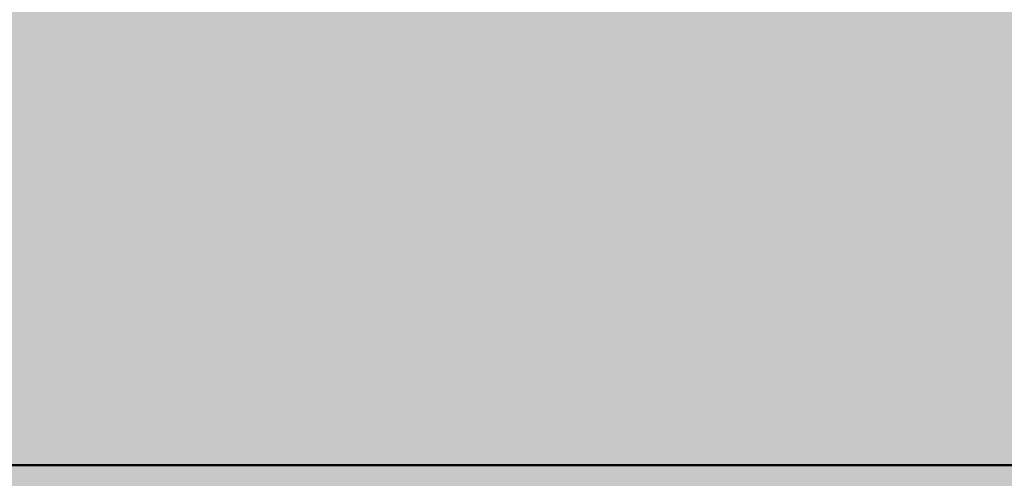
# Model space of a CAD drawing. Units: millimetres. Extents: x 0 to 2267, y 0 to 1823.
# Tile 147 of 256: x 1823.16 to 1833.61, y 1127.28 to 1132.15. Entities that reach past the tile are written whole.
import ezdxf

# ---------------------------------------------------------------- set-up
doc = ezdxf.new("R2010")
doc.units = ezdxf.units.MM
doc.header["$MEASUREMENT"] = 0
for name, color, linetype, lineweight in [('M-DIMS', 2, 'Continuous', 25), ('M-HATC', 252, 'Continuous', 18), ('M-OUTL', 7, 'Continuous', 50)]:
    doc.layers.add(name, color=color, linetype=linetype, lineweight=lineweight)
doc.styles.get("Standard").update_dxf_attribs({"font": 'arial.ttf'})
doc.dimstyles.get("Standard").update_dxf_attribs({"dimtxt": 7, "dimasz": 4, "dimexe": 0.18, "dimexo": 0.0625, "dimgap": 0.09, "dimtad": 0, "dimdec": 0, "dimzin": 0, "dimdsep": 46, "dimtxsty": 'Standard', "dimcen": 0.09, "dimadec": 0, "dimazin": 0, "dimtfac": 1, "dimtdec": 0, "dimtofl": 0, "dimtmove": 0, "dimatfit": 3, "dimfxl": 1, "dimtolj": 1, "dimtzin": 0, "dimarcsym": 0})

# ---------------------------------------------------------------- blocks, each defined once
blk = doc.blocks.new('*D1')
at = {"layer": 'Defpoints', "color": 0, "transparency": 16777216}
for p in [(1593.429, 1127.417), (1843.429, 1127.417), (1843.429, 955.628)]:
    blk.add_point(p, dxfattribs=at)
at = {"layer": 'M-DIMS', "color": 0, "lineweight": -2, "transparency": 16777216}
for p, q in [((1593.429, 1127.355), (1593.429, 955.448)), ((1843.429, 1127.355), (1843.429, 955.448)), ((1597.429, 955.628), (1710.558, 955.628)), ((1839.429, 955.628), (1726.3, 955.628))]:
    blk.add_line(p, q, dxfattribs=at)
at = {"layer": 'M-DIMS', "color": 0, "transparency": 16777216}
for points in [[(1597.429, 956.294), (1597.429, 954.961), (1593.429, 955.628)], [(1839.429, 956.294), (1839.429, 954.961), (1843.429, 955.628)]]:
    blk.add_solid(points, dxfattribs=at)
at = {"layer": 'M-DIMS', "color": 0, "transparency": 16777216, "insert": (1718.429, 955.628), "char_height": 7, "attachment_point": 5}
blk.add_mtext('\\A1;250', dxfattribs=at)

msp = doc.modelspace()

# ---------------------------------------------------------------- hatches: boundary and pattern name
at = {"layer": 'M-HATC'}
h = msp.add_hatch(color=256, dxfattribs=at)
h.dxf.hatch_style = 1
h.paths.add_polyline_path([(2055.771, 1603.062), (1381.087, 1603.062), (1381.087, 1598.062), (2055.771, 1598.062)])
h.paths.add_polyline_path([(2055.771, 1598.062), (1381.087, 1598.062), (1381.087, 1593.062), (2055.771, 1593.062)])
h.paths.add_polyline_path([(2051.307, 1536.761), (1385.55, 1536.761), (1385.55, 1526.761), (1387.55, 1526.761), (1388.537, 1525.053), (1385.332, 1521.233), (1385.332, 1521.223), (2050.254, 1522.749), (2048.321, 1525.053), (2049.307, 1526.761), (2051.307, 1526.761)])
edge = h.paths.add_edge_path()
edge.add_arc((1847.535, 1379.149), 135, 222.60306, 222.89085, ccw=False)
edge.add_line((1748.166, 1287.766), (1683.092, 1287.766))
edge.add_arc((1583.724, 1379.149), 135, 317.10915, 317.39694, ccw=False)
edge.add_arc((1678.969, 1290.671), 5, 222.8909, 317.1091, ccw=False)
edge.add_arc((1774.213, 1379.149), 135, 222.60306, 222.89085, ccw=False)
edge.add_line((1674.845, 1287.766), (1609.771, 1287.766))
edge.add_arc((1510.403, 1379.149), 135, 317.10915, 317.39694, ccw=False)
edge.add_arc((1605.647, 1290.671), 5, 222.8909, 317.1091, ccw=False)
edge.add_arc((1700.892, 1379.149), 135, 222.60306, 222.89085, ccw=False)
edge.add_line((1601.524, 1287.766), (1536.45, 1287.766))
edge.add_arc((1437.081, 1379.149), 135, 317.10915, 317.39694, ccw=False)
edge.add_arc((1532.326, 1290.671), 5, 222.8909, 317.1091, ccw=False)
edge.add_arc((1627.571, 1379.149), 135, 222.60306, 222.89085, ccw=False)
edge.add_line((1528.203, 1287.766), (1505.929, 1287.766))
edge.add_spline(control_points=[(1505.929, 1287.766), (1504.262, 1287.766), (1504.262, 1282.766), (1505.929, 1282.766)], knot_values=[0, 0, 0, 0, 5, 5, 5, 5], degree=3, periodic=0)
edge.add_line((1505.929, 1282.766), (1930.929, 1282.766))
edge.add_spline(control_points=[(1930.929, 1282.766), (1932.596, 1282.766), (1932.596, 1287.766), (1930.929, 1287.766)], knot_values=[0, 0, 0, 0, 5, 5, 5, 5], degree=3, periodic=0)
edge.add_line((1930.929, 1287.766), (1903.056, 1287.766))
edge.add_arc((1803.688, 1379.149), 135, 317.10915, 317.39694, ccw=False)
edge.add_arc((1898.932, 1290.671), 5, 222.8909, 317.1091, ccw=False)
edge.add_arc((1994.177, 1379.149), 135, 222.60306, 222.89085, ccw=False)
edge.add_line((1894.809, 1287.766), (1829.735, 1287.766))
edge.add_arc((1730.366, 1379.149), 135, 317.10915, 317.39694, ccw=False)
edge.add_arc((1825.611, 1290.671), 5, 222.8909, 317.1091, ccw=False)
edge.add_arc((1920.856, 1379.149), 135, 222.60306, 222.89085, ccw=False)
edge.add_line((1821.487, 1287.766), (1756.413, 1287.766))
edge.add_arc((1657.045, 1379.149), 135, 317.10915, 317.39694, ccw=False)
edge.add_arc((1752.29, 1290.671), 5, 222.8909, 317.1091, ccw=False)
edge = h.paths.add_edge_path()
edge.add_spline(control_points=[(1843.429, 1227.247), (1845.096, 1227.247), (1845.096, 1232.247), (1843.429, 1232.247)], knot_values=[0, 0, 0, 0, 5, 5, 5, 5], degree=3, periodic=0)
edge.add_line((1843.429, 1232.247), (1593.429, 1232.247))
edge.add_spline(control_points=[(1593.429, 1232.247), (1591.762, 1232.247), (1591.762, 1227.247), (1593.429, 1227.247)], knot_values=[0, 0, 0, 0, 5, 5, 5, 5], degree=3, periodic=0)
edge.add_line((1593.429, 1227.247), (1843.429, 1227.247))
h.paths.add_polyline_path([(1905.929, 1127.417), (1530.929, 1127.417, 0.414214), (1520.929, 1117.417), (1530.929, 1117.417), (1915.929, 1117.417, 0.414214)])
edge = h.paths.add_edge_path()
edge.add_arc((1397.086, 1498.408), 12.73, 90.7821, 190.8787, ccw=False)
edge.add_line((1396.912, 1511.136), (1428.01, 1511.349))
edge.add_line((1428.01, 1511.349), (1433.01, 1511.349))
edge.add_line((1433.01, 1511.349), (1434.439, 1511.349))
edge.add_arc((1419.474, 1498.08), 20, 41.561, 74.0821)
edge.add_line((1424.959, 1517.314), (1399.935, 1517.256))
edge.add_spline(control_points=[(1399.931, 1517.256), (1399.884, 1517.213), (1399.833, 1517.169), (1399.777, 1517.124)], knot_values=[11.567499, 11.567499, 11.567499, 11.567499, 11.814249, 11.814249, 11.814249, 11.814249], degree=3, periodic=0)
edge.add_spline(control_points=[(1399.633, 1517.01), (1399.583, 1516.972), (1399.531, 1516.934), (1399.476, 1516.895)], knot_values=[11.167718, 11.167718, 11.167718, 11.167718, 11.365188, 11.365188, 11.365188, 11.365188], degree=3, periodic=0)
edge.add_spline(control_points=[(1399.34, 1516.8), (1399.151, 1516.672), (1398.938, 1516.538), (1398.704, 1516.399)], knot_values=[10.376405, 10.376405, 10.376405, 10.376405, 11.00994, 11.00994, 11.00994, 11.00994], degree=3, periodic=0)
edge.add_spline(control_points=[(1398.657, 1516.372), (1398.579, 1516.326), (1398.498, 1516.28), (1398.415, 1516.233)], knot_values=[10.125175, 10.125175, 10.125175, 10.125175, 10.334406, 10.334406, 10.334406, 10.334406], degree=3, periodic=0)
edge.add_spline(control_points=[(1398.264, 1516.149), (1398.196, 1516.111), (1398.126, 1516.073), (1398.055, 1516.035)], knot_values=[9.832246, 9.832246, 9.832246, 9.832246, 9.999658, 9.999658, 9.999658, 9.999658], degree=3, periodic=0)
edge.add_spline(control_points=[(1397.999, 1516.005), (1397.731, 1515.862), (1397.446, 1515.717), (1397.147, 1515.571)], knot_values=[9.161808, 9.161808, 9.161808, 9.161808, 9.787769, 9.787769, 9.787769, 9.787769], degree=3, periodic=0)
edge.add_spline(control_points=[(1397.147, 1515.571), (1396.842, 1515.423), (1396.522, 1515.274), (1396.191, 1515.126)], knot_values=[8.524455, 8.524455, 8.524455, 8.524455, 9.161808, 9.161808, 9.161808, 9.161808], degree=3, periodic=0)
edge.add_spline(control_points=[(1396.078, 1515.076), (1395.985, 1515.035), (1395.892, 1514.994), (1395.798, 1514.953)], knot_values=[8.275193, 8.275193, 8.275193, 8.275193, 8.451726, 8.451726, 8.451726, 8.451726], degree=3, periodic=0)
edge.add_spline(control_points=[(1395.602, 1514.869), (1395.5, 1514.826), (1395.397, 1514.782), (1395.293, 1514.739)], knot_values=[7.962917, 7.962917, 7.962917, 7.962917, 8.152764, 8.152764, 8.152764, 8.152764], degree=3, periodic=0)
edge.add_spline(control_points=[(1395.212, 1514.706), (1394.828, 1514.547), (1394.435, 1514.393), (1394.036, 1514.244)], knot_values=[7.21254, 7.21254, 7.21254, 7.21254, 7.913148, 7.913148, 7.913148, 7.913148], degree=3, periodic=0)
edge.add_spline(control_points=[(1394.036, 1514.244), (1393.708, 1514.121), (1393.375, 1514.003), (1393.043, 1513.889)], knot_values=[6.633733, 6.633733, 6.633733, 6.633733, 7.21254, 7.21254, 7.21254, 7.21254], degree=3, periodic=0)
edge.add_spline(control_points=[(1392.821, 1513.815), (1392.72, 1513.781), (1392.618, 1513.748), (1392.517, 1513.715)], knot_values=[6.328796, 6.328796, 6.328796, 6.328796, 6.505493, 6.505493, 6.505493, 6.505493], degree=3, periodic=0)
edge.add_spline(control_points=[(1392.517, 1513.715), (1392.319, 1513.652), (1392.121, 1513.59), (1391.924, 1513.531)], knot_values=[5.984605, 5.984605, 5.984605, 5.984605, 6.328796, 6.328796, 6.328796, 6.328796], degree=3, periodic=0)
edge.add_spline(control_points=[(1391.792, 1513.491), (1391.312, 1513.35), (1390.838, 1513.224), (1390.378, 1513.117)], knot_values=[5.066697, 5.066697, 5.066697, 5.066697, 5.907055, 5.907055, 5.907055, 5.907055], degree=3, periodic=0)
edge.add_spline(control_points=[(1390.378, 1513.117), (1390.18, 1513.071), (1389.984, 1513.028), (1389.791, 1512.99)], knot_values=[4.70367, 4.70367, 4.70367, 4.70367, 5.066695, 5.066695, 5.066695, 5.066695], degree=3, periodic=0)
edge.add_spline(control_points=[(1389.422, 1512.92), (1389.246, 1512.889), (1389.073, 1512.862), (1388.904, 1512.838)], knot_values=[4.130571, 4.130571, 4.130571, 4.130571, 4.469816, 4.469816, 4.469816, 4.469816], degree=3, periodic=0)
edge.add_spline(control_points=[(1388.904, 1512.838), (1388.591, 1512.795), (1388.291, 1512.764), (1388.007, 1512.749)], knot_values=[3.504031, 3.504031, 3.504031, 3.504031, 4.130571, 4.130571, 4.130571, 4.130571], degree=3, periodic=0)
edge.add_spline(control_points=[(1387.936, 1512.746), (1387.854, 1512.742), (1387.773, 1512.74), (1387.694, 1512.739)], knot_values=[3.268866, 3.268866, 3.268866, 3.268866, 3.451164, 3.451164, 3.451164, 3.451164], degree=3, periodic=0)
edge.add_spline(control_points=[(1387.335, 1512.744), (1387.208, 1512.75), (1387.085, 1512.76), (1386.967, 1512.774)], knot_values=[2.670686, 2.670686, 2.670686, 2.670686, 2.984, 2.984, 2.984, 2.984], degree=3, periodic=0)
edge.add_spline(control_points=[(1386.833, 1512.792), (1386.821, 1512.794), (1386.809, 1512.796), (1386.797, 1512.798)], knot_values=[2.516981, 2.516981, 2.516981, 2.516981, 2.549528, 2.549528, 2.549528, 2.549528], degree=3, periodic=0)
edge.add_spline(control_points=[(1386.453, 1512.873), (1386.426, 1512.881), (1386.399, 1512.889), (1386.373, 1512.897)], knot_values=[2.095869, 2.095869, 2.095869, 2.095869, 2.17941, 2.17941, 2.17941, 2.17941], degree=3, periodic=0)
edge.add_spline(control_points=[(1386.069, 1513.019), (1386.063, 1513.022), (1386.058, 1513.025), (1386.052, 1513.028)], knot_values=[1.72453, 1.72453, 1.72453, 1.72453, 1.745933, 1.745933, 1.745933, 1.745933], degree=3, periodic=0)
edge.add_arc((1399.474, 1498.08), 20, 131.8243, 180)
edge.add_arc((1630.334, 1505.548), 250.971, 181.70518, 236.42798)
edge.add_arc((1605.34, 1483.304), 218.782, 238.66083, 243.34961)
edge.add_arc((1647.091, 1510.359), 262.899, 183.12984, 237.85344, ccw=False)
h.paths.add_polyline_path([(1406.537, 1391.964, 0.149382), (1491.551, 1296.442, -0.129517)], flags=17)
edge = h.paths.add_edge_path()
edge.add_arc((2037.384, 1498.08), 20, 0, 48.2659)
edge.add_spline(control_points=[(2050.697, 1513.005), (2050.651, 1512.985), (2050.603, 1512.966), (2050.554, 1512.948)], knot_values=[1.835652, 1.835652, 1.835652, 1.835652, 2.000781, 2.000781, 2.000781, 2.000781], degree=3, periodic=0)
edge.add_spline(control_points=[(2050.462, 1512.917), (2050.479, 1512.922), (2050.496, 1512.928), (2050.513, 1512.934)], knot_values=[2.045477, 2.045477, 2.045477, 2.045477, 2.101389, 2.101389, 2.101389, 2.101389], degree=3, periodic=0)
edge.add_spline(control_points=[(2050.129, 1512.834), (2050.198, 1512.847), (2050.266, 1512.862), (2050.331, 1512.879)], knot_values=[2.237629, 2.237629, 2.237629, 2.237629, 2.435841, 2.435841, 2.435841, 2.435841], degree=3, periodic=0)
edge.add_spline(control_points=[(2050.095, 1512.828), (2050.106, 1512.83), (2050.118, 1512.832), (2050.129, 1512.834)], knot_values=[2.435841, 2.435841, 2.435841, 2.435841, 2.468321, 2.468321, 2.468321, 2.468321], degree=3, periodic=0)
edge.add_spline(control_points=[(2049.784, 1512.785), (2049.855, 1512.792), (2049.924, 1512.801), (2049.992, 1512.811)], knot_values=[2.563852, 2.563852, 2.563852, 2.563852, 2.748541, 2.748541, 2.748541, 2.748541], degree=3, periodic=0)
edge.add_spline(control_points=[(2049.405, 1512.762), (2049.536, 1512.765), (2049.663, 1512.773), (2049.784, 1512.785)], knot_values=[2.748541, 2.748541, 2.748541, 2.748541, 3.064882, 3.064882, 3.064882, 3.064882], degree=3, periodic=0)
edge.add_spline(control_points=[(2049.17, 1512.76), (2049.234, 1512.759), (2049.297, 1512.759), (2049.358, 1512.761)], knot_values=[3.102309, 3.102309, 3.102309, 3.102309, 3.2503, 3.2503, 3.2503, 3.2503], degree=3, periodic=0)
edge.add_spline(control_points=[(2048.857, 1512.769), (2048.964, 1512.764), (2049.068, 1512.761), (2049.17, 1512.76)], knot_values=[3.2503, 3.2503, 3.2503, 3.2503, 3.486069, 3.486069, 3.486069, 3.486069], degree=3, periodic=0)
edge.add_spline(control_points=[(2048.692, 1512.779), (2048.373, 1512.801), (2048.035, 1512.841), (2047.682, 1512.897)], knot_values=[3.606429, 3.606429, 3.606429, 3.606429, 4.2989, 4.2989, 4.2989, 4.2989], degree=3, periodic=0)
edge.add_spline(control_points=[(2047.682, 1512.897), (2047.546, 1512.919), (2047.408, 1512.942), (2047.268, 1512.969)], knot_values=[4.2989, 4.2989, 4.2989, 4.2989, 4.565769, 4.565769, 4.565769, 4.565769], degree=3, periodic=0)
edge.add_spline(control_points=[(2047.268, 1512.969), (2047.145, 1512.991), (2047.021, 1513.016), (2046.895, 1513.042)], knot_values=[4.565769, 4.565769, 4.565769, 4.565769, 4.799971, 4.799971, 4.799971, 4.799971], degree=3, periodic=0)
edge.add_spline(control_points=[(2046.895, 1513.042), (2046.529, 1513.119), (2046.151, 1513.209), (2045.768, 1513.311)], knot_values=[4.799971, 4.799971, 4.799971, 4.799971, 5.483718, 5.483718, 5.483718, 5.483718], degree=3, periodic=0)
edge.add_spline(control_points=[(2045.768, 1513.311), (2045.372, 1513.415), (2044.97, 1513.532), (2044.566, 1513.659)], knot_values=[5.483718, 5.483718, 5.483718, 5.483718, 6.187866, 6.187866, 6.187866, 6.187866], degree=3, periodic=0)
edge.add_spline(control_points=[(2044.566, 1513.659), (2044.415, 1513.706), (2044.263, 1513.755), (2044.112, 1513.805)], knot_values=[6.187866, 6.187866, 6.187866, 6.187866, 6.451551, 6.451551, 6.451551, 6.451551], degree=3, periodic=0)
edge.add_spline(control_points=[(2044.112, 1513.805), (2043.997, 1513.843), (2043.882, 1513.881), (2043.767, 1513.92)], knot_values=[6.451551, 6.451551, 6.451551, 6.451551, 6.651434, 6.651434, 6.651434, 6.651434], degree=3, periodic=0)
edge.add_spline(control_points=[(2043.767, 1513.92), (2043.372, 1514.055), (2042.977, 1514.198), (2042.589, 1514.346)], knot_values=[6.651434, 6.651434, 6.651434, 6.651434, 7.338879, 7.338879, 7.338879, 7.338879], degree=3, periodic=0)
edge.add_spline(control_points=[(2042.589, 1514.346), (2042.164, 1514.507), (2041.746, 1514.675), (2041.341, 1514.846)], knot_values=[7.338879, 7.338879, 7.338879, 7.338879, 8.089209, 8.089209, 8.089209, 8.089209], degree=3, periodic=0)
edge.add_spline(control_points=[(2041.341, 1514.846), (2041.103, 1514.946), (2040.869, 1515.048), (2040.64, 1515.15)], knot_values=[8.089209, 8.089209, 8.089209, 8.089209, 8.529587, 8.529587, 8.529587, 8.529587], degree=3, periodic=0)
edge.add_spline(control_points=[(2040.51, 1515.209), (2040.082, 1515.402), (2039.675, 1515.597), (2039.295, 1515.789)], knot_values=[8.613818, 8.613818, 8.613818, 8.613818, 9.44571, 9.44571, 9.44571, 9.44571], degree=3, periodic=0)
edge.add_spline(control_points=[(2039.295, 1515.789), (2039.062, 1515.907), (2038.839, 1516.025), (2038.629, 1516.14)], knot_values=[9.44571, 9.44571, 9.44571, 9.44571, 9.956404, 9.956404, 9.956404, 9.956404], degree=3, periodic=0)
edge.add_spline(control_points=[(2038.629, 1516.14), (2038.519, 1516.2), (2038.412, 1516.26), (2038.309, 1516.319)], knot_values=[9.956404, 9.956404, 9.956404, 9.956404, 10.223542, 10.223542, 10.223542, 10.223542], degree=3, periodic=0)
edge.add_spline(control_points=[(2038.309, 1516.319), (2038.214, 1516.374), (2038.122, 1516.428), (2038.033, 1516.481)], knot_values=[10.223542, 10.223542, 10.223542, 10.223542, 10.47051, 10.47051, 10.47051, 10.47051], degree=3, periodic=0)
edge.add_spline(control_points=[(2038.033, 1516.481), (2037.786, 1516.63), (2037.564, 1516.773), (2037.372, 1516.909)], knot_values=[10.47051, 10.47051, 10.47051, 10.47051, 11.15767, 11.15767, 11.15767, 11.15767], degree=3, periodic=0)
edge.add_spline(control_points=[(2037.372, 1516.909), (2037.279, 1516.975), (2037.193, 1517.04), (2037.114, 1517.102)], knot_values=[11.15767, 11.15767, 11.15767, 11.15767, 11.49227, 11.49227, 11.49227, 11.49227], degree=3, periodic=0)
edge.add_spline(control_points=[(2036.856, 1517.326), (2036.915, 1517.269), (2036.981, 1517.21), (2037.056, 1517.149)], knot_values=[11.577341, 11.577341, 11.577341, 11.577341, 11.91035, 11.91035, 11.91035, 11.91035], degree=3, periodic=0)
edge.add_spline(control_points=[(2036.807, 1517.375), (2036.823, 1517.359), (2036.839, 1517.342), (2036.856, 1517.326)], knot_values=[11.91035, 11.91035, 11.91035, 11.91035, 12.007402, 12.007402, 12.007402, 12.007402], degree=3, periodic=0)
edge.add_spline(control_points=[(2036.702, 1517.494), (2036.71, 1517.483), (2036.72, 1517.472), (2036.729, 1517.461)], knot_values=[12.184155, 12.184155, 12.184155, 12.184155, 12.255409, 12.255409, 12.255409, 12.255409], degree=3, periodic=0)
edge.add_spline(control_points=[(2036.616, 1517.621), (2036.62, 1517.613), (2036.624, 1517.606), (2036.629, 1517.598)], knot_values=[12.487913, 12.487913, 12.487913, 12.487913, 12.541035, 12.541035, 12.541035, 12.541035], degree=3, periodic=0)
edge.add_spline(control_points=[(2036.563, 1517.786), (2036.564, 1517.779), (2036.564, 1517.773), (2036.565, 1517.766)], knot_values=[12.911761, 12.911761, 12.911761, 12.911761, 12.968286, 12.968286, 12.968286, 12.968286], degree=3, periodic=0)
edge.add_spline(control_points=[(2036.617, 1517.93), (2036.612, 1517.926), (2036.609, 1517.921), (2036.605, 1517.916)], knot_values=[13.382527, 13.382527, 13.382527, 13.382527, 13.433791, 13.433791, 13.433791, 13.433791], degree=3, periodic=0)
edge.add_spline(control_points=[(2036.749, 1518.017), (2036.736, 1518.012), (2036.724, 1518.006), (2036.712, 1518)], knot_values=[13.726299, 13.726299, 13.726299, 13.726299, 13.809928, 13.809928, 13.809928, 13.809928], degree=3, periodic=0)
edge.add_spline(control_points=[(2036.86, 1518.053), (2036.839, 1518.047), (2036.818, 1518.042), (2036.799, 1518.035)], knot_values=[13.910887, 13.910887, 13.910887, 13.910887, 14.02153, 14.02153, 14.02153, 14.02153], degree=3, periodic=0)
edge.add_line((2036.964, 1518.08), (2032.384, 1518.08))
edge.add_line((2032.384, 1518.08), (2027.384, 1518.08))
edge.add_line((2027.384, 1518.08), (2022.384, 1518.08))
edge.add_line((2022.384, 1518.08), (2017.384, 1518.08))
edge.add_arc((2017.384, 1498.08), 20, 90, 138.439)
edge.add_line((2002.419, 1511.349), (2003.848, 1511.349))
edge.add_line((2003.848, 1511.349), (2008.848, 1511.349))
edge.add_line((2008.848, 1511.349), (2039.772, 1511.138))
edge.add_arc((2039.772, 1498.408), 12.73, -10.8787, 90, ccw=False)
edge.add_arc((1789.767, 1510.359), 262.899, 302.14656, 356.87016, ccw=False)
edge.add_arc((1831.518, 1483.304), 218.782, 296.65039, 301.33917)
edge.add_arc((1806.524, 1505.548), 250.971, 303.57202, 358.29482)
h.paths.add_polyline_path([(2030.321, 1391.964, -0.129517), (1945.307, 1296.442, 0.149382)], flags=17)
edge = h.paths.add_edge_path()
edge.add_spline(control_points=[(2037.246, 1518.082), (2037.29, 1518.081), (2037.336, 1518.08), (2037.384, 1518.08)], knot_values=[0.000012, 0.000012, 0.000012, 0.000012, 0.144754, 0.144754, 0.144754, 0.144754], degree=3, periodic=0)
edge.add_line((2037.336, 1518.08), (2037.01, 1518.08))
edge.add_spline(control_points=[(2037.01, 1518.08), (2036.982, 1518.077), (2036.956, 1518.073), (2036.931, 1518.068)], knot_values=[14.13465, 14.13465, 14.13465, 14.13465, 14.247197, 14.247197, 14.247197, 14.247197], degree=3, periodic=0)
edge.add_spline(control_points=[(2036.931, 1518.068), (2036.928, 1518.067), (2036.924, 1518.067), (2036.921, 1518.066)], knot_values=[14.118315, 14.118315, 14.118315, 14.118315, 14.13465, 14.13465, 14.13465, 14.13465], degree=3, periodic=0)
edge.add_spline(control_points=[(2036.921, 1518.066), (2036.912, 1518.064), (2036.903, 1518.063), (2036.895, 1518.061)], knot_values=[14.078086, 14.078086, 14.078086, 14.078086, 14.118315, 14.118315, 14.118315, 14.118315], degree=3, periodic=0)
edge.add_spline(control_points=[(2036.895, 1518.061), (2036.883, 1518.058), (2036.872, 1518.056), (2036.86, 1518.053)], knot_values=[14.02153, 14.02153, 14.02153, 14.02153, 14.078086, 14.078086, 14.078086, 14.078086], degree=3, periodic=0)
edge.add_spline(control_points=[(2036.86, 1518.053), (2036.839, 1518.047), (2036.818, 1518.042), (2036.799, 1518.035)], knot_values=[13.910887, 13.910887, 13.910887, 13.910887, 14.02153, 14.02153, 14.02153, 14.02153], degree=3, periodic=0)
edge.add_spline(control_points=[(2036.799, 1518.035), (2036.798, 1518.035), (2036.797, 1518.035), (2036.797, 1518.035)], knot_values=[13.906906, 13.906906, 13.906906, 13.906906, 13.910887, 13.910887, 13.910887, 13.910887], degree=3, periodic=0)
edge.add_spline(control_points=[(2036.797, 1518.035), (2036.788, 1518.032), (2036.78, 1518.029), (2036.772, 1518.026)], knot_values=[13.857826, 13.857826, 13.857826, 13.857826, 13.906906, 13.906906, 13.906906, 13.906906], degree=3, periodic=0)
edge.add_spline(control_points=[(2036.772, 1518.026), (2036.764, 1518.023), (2036.756, 1518.02), (2036.749, 1518.017)], knot_values=[13.809928, 13.809928, 13.809928, 13.809928, 13.857826, 13.857826, 13.857826, 13.857826], degree=3, periodic=0)
edge.add_spline(control_points=[(2036.749, 1518.017), (2036.736, 1518.012), (2036.724, 1518.006), (2036.712, 1518)], knot_values=[13.726299, 13.726299, 13.726299, 13.726299, 13.809928, 13.809928, 13.809928, 13.809928], degree=3, periodic=0)
edge.add_spline(control_points=[(2036.712, 1518), (2036.712, 1518), (2036.712, 1518), (2036.711, 1518)], knot_values=[13.723993, 13.723993, 13.723993, 13.723993, 13.726299, 13.726299, 13.726299, 13.726299], degree=3, periodic=0)
edge.add_spline(control_points=[(2036.711, 1518), (2036.706, 1517.997), (2036.701, 1517.994), (2036.696, 1517.992)], knot_values=[13.686536, 13.686536, 13.686536, 13.686536, 13.723993, 13.723993, 13.723993, 13.723993], degree=3, periodic=0)
edge.add_spline(control_points=[(2036.696, 1517.992), (2036.692, 1517.989), (2036.687, 1517.987), (2036.683, 1517.984)], knot_values=[13.651251, 13.651251, 13.651251, 13.651251, 13.686536, 13.686536, 13.686536, 13.686536], degree=3, periodic=0)
edge.add_spline(control_points=[(2036.683, 1517.984), (2036.676, 1517.98), (2036.67, 1517.976), (2036.664, 1517.971)], knot_values=[13.596804, 13.596804, 13.596804, 13.596804, 13.651251, 13.651251, 13.651251, 13.651251], degree=3, periodic=0)
edge.add_spline(control_points=[(2036.664, 1517.971), (2036.664, 1517.971), (2036.663, 1517.971), (2036.663, 1517.971)], knot_values=[13.593956, 13.593956, 13.593956, 13.593956, 13.596804, 13.596804, 13.596804, 13.596804], degree=3, periodic=0)
edge.add_spline(control_points=[(2036.663, 1517.971), (2036.66, 1517.969), (2036.658, 1517.967), (2036.655, 1517.965)], knot_values=[13.570322, 13.570322, 13.570322, 13.570322, 13.593956, 13.593956, 13.593956, 13.593956], degree=3, periodic=0)
edge.add_spline(control_points=[(2036.655, 1517.965), (2036.653, 1517.963), (2036.65, 1517.961), (2036.647, 1517.959)], knot_values=[13.545477, 13.545477, 13.545477, 13.545477, 13.570322, 13.570322, 13.570322, 13.570322], degree=3, periodic=0)
edge.add_spline(control_points=[(2036.647, 1517.959), (2036.647, 1517.959), (2036.647, 1517.959), (2036.647, 1517.959)], knot_values=[13.543931, 13.543931, 13.543931, 13.543931, 13.545477, 13.545477, 13.545477, 13.545477], degree=3, periodic=0)
edge.add_spline(control_points=[(2036.647, 1517.959), (2036.641, 1517.954), (2036.636, 1517.949), (2036.631, 1517.945)], knot_values=[13.488237, 13.488237, 13.488237, 13.488237, 13.543931, 13.543931, 13.543931, 13.543931], degree=3, periodic=0)
edge.add_spline(control_points=[(2036.631, 1517.945), (2036.628, 1517.942), (2036.626, 1517.94), (2036.623, 1517.937)], knot_values=[13.460307, 13.460307, 13.460307, 13.460307, 13.488237, 13.488237, 13.488237, 13.488237], degree=3, periodic=0)
edge.add_spline(control_points=[(2036.623, 1517.937), (2036.622, 1517.936), (2036.62, 1517.934), (2036.618, 1517.932)], knot_values=[13.439712, 13.439712, 13.439712, 13.439712, 13.460307, 13.460307, 13.460307, 13.460307], degree=3, periodic=0)
edge.add_spline(control_points=[(2036.618, 1517.932), (2036.618, 1517.931), (2036.617, 1517.931), (2036.617, 1517.93)], knot_values=[13.433791, 13.433791, 13.433791, 13.433791, 13.439712, 13.439712, 13.439712, 13.439712], degree=3, periodic=0)
edge.add_spline(control_points=[(2036.617, 1517.93), (2036.612, 1517.926), (2036.609, 1517.921), (2036.605, 1517.916)], knot_values=[13.382527, 13.382527, 13.382527, 13.382527, 13.433791, 13.433791, 13.433791, 13.433791], degree=3, periodic=0)
edge.add_spline(control_points=[(2036.605, 1517.916), (2036.603, 1517.913), (2036.6, 1517.91), (2036.598, 1517.907)], knot_values=[13.350017, 13.350017, 13.350017, 13.350017, 13.382527, 13.382527, 13.382527, 13.382527], degree=3, periodic=0)
edge.add_spline(control_points=[(2036.598, 1517.907), (2036.597, 1517.906), (2036.596, 1517.904), (2036.595, 1517.903)], knot_values=[13.333922, 13.333922, 13.333922, 13.333922, 13.350017, 13.350017, 13.350017, 13.350017], degree=3, periodic=0)
edge.add_spline(control_points=[(2036.595, 1517.903), (2036.595, 1517.902), (2036.594, 1517.901), (2036.593, 1517.9)], knot_values=[13.323828, 13.323828, 13.323828, 13.323828, 13.333922, 13.333922, 13.333922, 13.333922], degree=3, periodic=0)
edge.add_spline(control_points=[(2036.593, 1517.9), (2036.59, 1517.895), (2036.588, 1517.891), (2036.585, 1517.886)], knot_values=[13.277545, 13.277545, 13.277545, 13.277545, 13.323828, 13.323828, 13.323828, 13.323828], degree=3, periodic=0)
edge.add_spline(control_points=[(2036.585, 1517.886), (2036.584, 1517.883), (2036.582, 1517.879), (2036.58, 1517.875)], knot_values=[13.240119, 13.240119, 13.240119, 13.240119, 13.277545, 13.277545, 13.277545, 13.277545], degree=3, periodic=0)
edge.add_spline(control_points=[(2036.58, 1517.875), (2036.58, 1517.874), (2036.579, 1517.873), (2036.578, 1517.872)], knot_values=[13.228211, 13.228211, 13.228211, 13.228211, 13.240119, 13.240119, 13.240119, 13.240119], degree=3, periodic=0)
edge.add_spline(control_points=[(2036.578, 1517.872), (2036.578, 1517.87), (2036.577, 1517.869), (2036.577, 1517.868)], knot_values=[13.215717, 13.215717, 13.215717, 13.215717, 13.228211, 13.228211, 13.228211, 13.228211], degree=3, periodic=0)
edge.add_spline(control_points=[(2036.577, 1517.868), (2036.575, 1517.864), (2036.574, 1517.86), (2036.573, 1517.857)], knot_values=[13.179847, 13.179847, 13.179847, 13.179847, 13.215717, 13.215717, 13.215717, 13.215717], degree=3, periodic=0)
edge.add_spline(control_points=[(2036.573, 1517.857), (2036.571, 1517.851), (2036.57, 1517.846), (2036.569, 1517.841)], knot_values=[13.132017, 13.132017, 13.132017, 13.132017, 13.179847, 13.179847, 13.179847, 13.179847], degree=3, periodic=0)
edge.add_spline(control_points=[(2036.569, 1517.841), (2036.568, 1517.84), (2036.568, 1517.839), (2036.568, 1517.838)], knot_values=[13.122482, 13.122482, 13.122482, 13.122482, 13.132017, 13.132017, 13.132017, 13.132017], degree=3, periodic=0)
edge.add_spline(control_points=[(2036.568, 1517.838), (2036.568, 1517.836), (2036.567, 1517.835), (2036.567, 1517.833)], knot_values=[13.105592, 13.105592, 13.105592, 13.105592, 13.122482, 13.122482, 13.122482, 13.122482], degree=3, periodic=0)
edge.add_spline(control_points=[(2036.567, 1517.833), (2036.566, 1517.829), (2036.566, 1517.826), (2036.565, 1517.822)], knot_values=[13.074063, 13.074063, 13.074063, 13.074063, 13.105592, 13.105592, 13.105592, 13.105592], degree=3, periodic=0)
edge.add_spline(control_points=[(2036.565, 1517.822), (2036.565, 1517.822), (2036.565, 1517.822), (2036.565, 1517.822)], knot_values=[13.074043, 13.074043, 13.074043, 13.074043, 13.074063, 13.074063, 13.074063, 13.074063], degree=3, periodic=0)
edge.add_spline(control_points=[(2036.565, 1517.822), (2036.564, 1517.816), (2036.564, 1517.811), (2036.564, 1517.805)], knot_values=[13.021884, 13.021884, 13.021884, 13.021884, 13.074043, 13.074043, 13.074043, 13.074043], degree=3, periodic=0)
edge.add_spline(control_points=[(2036.564, 1517.805), (2036.564, 1517.804), (2036.564, 1517.803), (2036.564, 1517.803)], knot_values=[13.01674, 13.01674, 13.01674, 13.01674, 13.021884, 13.021884, 13.021884, 13.021884], degree=3, periodic=0)
edge.add_spline(control_points=[(2036.564, 1517.803), (2036.563, 1517.801), (2036.563, 1517.798), (2036.563, 1517.796)], knot_values=[12.996438, 12.996438, 12.996438, 12.996438, 13.01674, 13.01674, 13.01674, 13.01674], degree=3, periodic=0)
edge.add_spline(control_points=[(2036.563, 1517.796), (2036.563, 1517.793), (2036.563, 1517.789), (2036.563, 1517.786)], knot_values=[12.968286, 12.968286, 12.968286, 12.968286, 12.996438, 12.996438, 12.996438, 12.996438], degree=3, periodic=0)
edge.add_spline(control_points=[(2036.563, 1517.786), (2036.564, 1517.779), (2036.564, 1517.773), (2036.565, 1517.766)], knot_values=[12.911761, 12.911761, 12.911761, 12.911761, 12.968286, 12.968286, 12.968286, 12.968286], degree=3, periodic=0)
edge.add_spline(control_points=[(2036.565, 1517.766), (2036.565, 1517.766), (2036.565, 1517.766), (2036.565, 1517.766)], knot_values=[12.911017, 12.911017, 12.911017, 12.911017, 12.911761, 12.911761, 12.911761, 12.911761], degree=3, periodic=0)
edge.add_spline(control_points=[(2036.565, 1517.766), (2036.565, 1517.762), (2036.566, 1517.759), (2036.566, 1517.756)], knot_values=[12.88528, 12.88528, 12.88528, 12.88528, 12.911017, 12.911017, 12.911017, 12.911017], degree=3, periodic=0)
edge.add_spline(control_points=[(2036.566, 1517.756), (2036.567, 1517.753), (2036.567, 1517.751), (2036.568, 1517.748)], knot_values=[12.862519, 12.862519, 12.862519, 12.862519, 12.88528, 12.88528, 12.88528, 12.88528], degree=3, periodic=0)
edge.add_spline(control_points=[(2036.568, 1517.748), (2036.568, 1517.747), (2036.568, 1517.747), (2036.568, 1517.746)], knot_values=[12.858885, 12.858885, 12.858885, 12.858885, 12.862519, 12.862519, 12.862519, 12.862519], degree=3, periodic=0)
edge.add_spline(control_points=[(2036.568, 1517.746), (2036.569, 1517.74), (2036.571, 1517.733), (2036.572, 1517.726)], knot_values=[12.8053, 12.8053, 12.8053, 12.8053, 12.858885, 12.858885, 12.858885, 12.858885], degree=3, periodic=0)
edge.add_spline(control_points=[(2036.572, 1517.726), (2036.573, 1517.723), (2036.574, 1517.719), (2036.576, 1517.715)], knot_values=[12.775176, 12.775176, 12.775176, 12.775176, 12.8053, 12.8053, 12.8053, 12.8053], degree=3, periodic=0)
edge.add_spline(control_points=[(2036.576, 1517.715), (2036.576, 1517.713), (2036.577, 1517.71), (2036.578, 1517.708)], knot_values=[12.756759, 12.756759, 12.756759, 12.756759, 12.775176, 12.775176, 12.775176, 12.775176], degree=3, periodic=0)
edge.add_spline(control_points=[(2036.578, 1517.708), (2036.578, 1517.707), (2036.578, 1517.706), (2036.579, 1517.705)], knot_values=[12.748742, 12.748742, 12.748742, 12.748742, 12.756759, 12.756759, 12.756759, 12.756759], degree=3, periodic=0)
edge.add_spline(control_points=[(2036.579, 1517.705), (2036.581, 1517.698), (2036.583, 1517.692), (2036.586, 1517.685)], knot_values=[12.69959, 12.69959, 12.69959, 12.69959, 12.748742, 12.748742, 12.748742, 12.748742], degree=3, periodic=0)
edge.add_spline(control_points=[(2036.586, 1517.685), (2036.588, 1517.68), (2036.59, 1517.675), (2036.592, 1517.669)], knot_values=[12.659038, 12.659038, 12.659038, 12.659038, 12.69959, 12.69959, 12.69959, 12.69959], degree=3, periodic=0)
edge.add_spline(control_points=[(2036.592, 1517.669), (2036.594, 1517.665), (2036.596, 1517.66), (2036.598, 1517.656)], knot_values=[12.626806, 12.626806, 12.626806, 12.626806, 12.659038, 12.659038, 12.659038, 12.659038], degree=3, periodic=0)
edge.add_spline(control_points=[(2036.598, 1517.656), (2036.598, 1517.655), (2036.599, 1517.654), (2036.599, 1517.653)], knot_values=[12.619394, 12.619394, 12.619394, 12.619394, 12.626806, 12.626806, 12.626806, 12.626806], degree=3, periodic=0)
edge.add_spline(control_points=[(2036.599, 1517.653), (2036.604, 1517.642), (2036.61, 1517.632), (2036.616, 1517.621)], knot_values=[12.541039, 12.541039, 12.541039, 12.541039, 12.619394, 12.619394, 12.619394, 12.619394], degree=3, periodic=0)
edge.add_spline(control_points=[(2036.616, 1517.621), (2036.616, 1517.621), (2036.616, 1517.621), (2036.616, 1517.621)], knot_values=[12.541035, 12.541035, 12.541035, 12.541035, 12.541039, 12.541039, 12.541039, 12.541039], degree=3, periodic=0)
edge.add_spline(control_points=[(2036.616, 1517.621), (2036.62, 1517.613), (2036.624, 1517.606), (2036.629, 1517.598)], knot_values=[12.487913, 12.487913, 12.487913, 12.487913, 12.541035, 12.541035, 12.541035, 12.541035], degree=3, periodic=0)
edge.add_spline(control_points=[(2036.629, 1517.598), (2036.633, 1517.592), (2036.637, 1517.585), (2036.641, 1517.579)], knot_values=[12.443982, 12.443982, 12.443982, 12.443982, 12.487913, 12.487913, 12.487913, 12.487913], degree=3, periodic=0)
edge.add_spline(control_points=[(2036.641, 1517.579), (2036.641, 1517.578), (2036.642, 1517.576), (2036.643, 1517.575)], knot_values=[12.434996, 12.434996, 12.434996, 12.434996, 12.443982, 12.443982, 12.443982, 12.443982], degree=3, periodic=0)
edge.add_spline(control_points=[(2036.643, 1517.575), (2036.653, 1517.56), (2036.664, 1517.544), (2036.676, 1517.528)], knot_values=[12.329647, 12.329647, 12.329647, 12.329647, 12.434996, 12.434996, 12.434996, 12.434996], degree=3, periodic=0)
edge.add_spline(control_points=[(2036.676, 1517.528), (2036.684, 1517.517), (2036.693, 1517.505), (2036.702, 1517.494)], knot_values=[12.255409, 12.255409, 12.255409, 12.255409, 12.329647, 12.329647, 12.329647, 12.329647], degree=3, periodic=0)
edge.add_spline(control_points=[(2036.702, 1517.494), (2036.71, 1517.483), (2036.72, 1517.472), (2036.729, 1517.461)], knot_values=[12.184155, 12.184155, 12.184155, 12.184155, 12.255409, 12.255409, 12.255409, 12.255409], degree=3, periodic=0)
edge.add_spline(control_points=[(2036.729, 1517.461), (2036.744, 1517.444), (2036.759, 1517.426), (2036.775, 1517.409)], knot_values=[12.075961, 12.075961, 12.075961, 12.075961, 12.184155, 12.184155, 12.184155, 12.184155], degree=3, periodic=0)
edge.add_spline(control_points=[(2036.775, 1517.409), (2036.776, 1517.407), (2036.777, 1517.406), (2036.778, 1517.405)], knot_values=[12.069502, 12.069502, 12.069502, 12.069502, 12.075961, 12.075961, 12.075961, 12.075961], degree=3, periodic=0)
edge.add_spline(control_points=[(2036.778, 1517.405), (2036.788, 1517.395), (2036.797, 1517.385), (2036.807, 1517.375)], knot_values=[12.007402, 12.007402, 12.007402, 12.007402, 12.069502, 12.069502, 12.069502, 12.069502], degree=3, periodic=0)
edge.add_spline(control_points=[(2036.807, 1517.375), (2036.823, 1517.359), (2036.839, 1517.342), (2036.856, 1517.326)], knot_values=[11.91035, 11.91035, 11.91035, 11.91035, 12.007402, 12.007402, 12.007402, 12.007402], degree=3, periodic=0)
edge.add_spline(control_points=[(2036.856, 1517.326), (2036.915, 1517.269), (2036.981, 1517.21), (2037.056, 1517.149)], knot_values=[11.577341, 11.577341, 11.577341, 11.577341, 11.91035, 11.91035, 11.91035, 11.91035], degree=3, periodic=0)
edge.add_spline(control_points=[(2037.056, 1517.149), (2037.075, 1517.134), (2037.094, 1517.118), (2037.114, 1517.102)], knot_values=[11.49227, 11.49227, 11.49227, 11.49227, 11.577341, 11.577341, 11.577341, 11.577341], degree=3, periodic=0)
edge.add_spline(control_points=[(2037.114, 1517.102), (2037.193, 1517.04), (2037.279, 1516.975), (2037.372, 1516.909)], knot_values=[11.15767, 11.15767, 11.15767, 11.15767, 11.49227, 11.49227, 11.49227, 11.49227], degree=3, periodic=0)
edge.add_spline(control_points=[(2037.372, 1516.909), (2037.564, 1516.773), (2037.786, 1516.63), (2038.033, 1516.481)], knot_values=[10.47051, 10.47051, 10.47051, 10.47051, 11.15767, 11.15767, 11.15767, 11.15767], degree=3, periodic=0)
edge.add_spline(control_points=[(2038.033, 1516.481), (2038.122, 1516.428), (2038.214, 1516.374), (2038.309, 1516.319)], knot_values=[10.223542, 10.223542, 10.223542, 10.223542, 10.47051, 10.47051, 10.47051, 10.47051], degree=3, periodic=0)
edge.add_spline(control_points=[(2038.309, 1516.319), (2038.412, 1516.26), (2038.519, 1516.2), (2038.629, 1516.14)], knot_values=[9.956404, 9.956404, 9.956404, 9.956404, 10.223542, 10.223542, 10.223542, 10.223542], degree=3, periodic=0)
edge.add_spline(control_points=[(2038.629, 1516.14), (2038.839, 1516.025), (2039.062, 1515.907), (2039.295, 1515.789)], knot_values=[9.44571, 9.44571, 9.44571, 9.44571, 9.956404, 9.956404, 9.956404, 9.956404], degree=3, periodic=0)
edge.add_spline(control_points=[(2039.295, 1515.789), (2039.675, 1515.597), (2040.082, 1515.402), (2040.51, 1515.209)], knot_values=[8.613818, 8.613818, 8.613818, 8.613818, 9.44571, 9.44571, 9.44571, 9.44571], degree=3, periodic=0)
edge.add_spline(control_points=[(2040.51, 1515.209), (2040.553, 1515.189), (2040.597, 1515.17), (2040.64, 1515.15)], knot_values=[8.529587, 8.529587, 8.529587, 8.529587, 8.613818, 8.613818, 8.613818, 8.613818], degree=3, periodic=0)
edge.add_spline(control_points=[(2040.64, 1515.15), (2040.869, 1515.048), (2041.103, 1514.946), (2041.341, 1514.846)], knot_values=[8.089209, 8.089209, 8.089209, 8.089209, 8.529587, 8.529587, 8.529587, 8.529587], degree=3, periodic=0)
edge.add_spline(control_points=[(2041.341, 1514.846), (2041.746, 1514.675), (2042.164, 1514.507), (2042.589, 1514.346)], knot_values=[7.338879, 7.338879, 7.338879, 7.338879, 8.089209, 8.089209, 8.089209, 8.089209], degree=3, periodic=0)
edge.add_spline(control_points=[(2042.589, 1514.346), (2042.977, 1514.198), (2043.372, 1514.055), (2043.767, 1513.92)], knot_values=[6.651434, 6.651434, 6.651434, 6.651434, 7.338879, 7.338879, 7.338879, 7.338879], degree=3, periodic=0)
edge.add_spline(control_points=[(2043.767, 1513.92), (2043.882, 1513.881), (2043.997, 1513.843), (2044.112, 1513.805)], knot_values=[6.451551, 6.451551, 6.451551, 6.451551, 6.651434, 6.651434, 6.651434, 6.651434], degree=3, periodic=0)
edge.add_spline(control_points=[(2044.112, 1513.805), (2044.263, 1513.755), (2044.415, 1513.706), (2044.566, 1513.659)], knot_values=[6.187866, 6.187866, 6.187866, 6.187866, 6.451551, 6.451551, 6.451551, 6.451551], degree=3, periodic=0)
edge.add_spline(control_points=[(2044.566, 1513.659), (2044.97, 1513.532), (2045.372, 1513.415), (2045.768, 1513.311)], knot_values=[5.483718, 5.483718, 5.483718, 5.483718, 6.187866, 6.187866, 6.187866, 6.187866], degree=3, periodic=0)
edge.add_spline(control_points=[(2045.768, 1513.311), (2046.151, 1513.209), (2046.529, 1513.119), (2046.895, 1513.042)], knot_values=[4.799971, 4.799971, 4.799971, 4.799971, 5.483718, 5.483718, 5.483718, 5.483718], degree=3, periodic=0)
edge.add_spline(control_points=[(2046.895, 1513.042), (2047.021, 1513.016), (2047.145, 1512.991), (2047.268, 1512.969)], knot_values=[4.565769, 4.565769, 4.565769, 4.565769, 4.799971, 4.799971, 4.799971, 4.799971], degree=3, periodic=0)
edge.add_spline(control_points=[(2047.268, 1512.969), (2047.408, 1512.942), (2047.546, 1512.919), (2047.682, 1512.897)], knot_values=[4.2989, 4.2989, 4.2989, 4.2989, 4.565769, 4.565769, 4.565769, 4.565769], degree=3, periodic=0)
edge.add_spline(control_points=[(2047.682, 1512.897), (2048.035, 1512.841), (2048.373, 1512.801), (2048.692, 1512.779)], knot_values=[3.606429, 3.606429, 3.606429, 3.606429, 4.2989, 4.2989, 4.2989, 4.2989], degree=3, periodic=0)
edge.add_spline(control_points=[(2048.692, 1512.779), (2048.748, 1512.775), (2048.803, 1512.772), (2048.857, 1512.769)], knot_values=[3.486069, 3.486069, 3.486069, 3.486069, 3.606429, 3.606429, 3.606429, 3.606429], degree=3, periodic=0)
edge.add_spline(control_points=[(2048.857, 1512.769), (2048.964, 1512.764), (2049.068, 1512.761), (2049.17, 1512.76)], knot_values=[3.2503, 3.2503, 3.2503, 3.2503, 3.486069, 3.486069, 3.486069, 3.486069], degree=3, periodic=0)
edge.add_spline(control_points=[(2049.17, 1512.76), (2049.234, 1512.759), (2049.297, 1512.759), (2049.358, 1512.761)], knot_values=[3.102309, 3.102309, 3.102309, 3.102309, 3.2503, 3.2503, 3.2503, 3.2503], degree=3, periodic=0)
edge.add_spline(control_points=[(2049.358, 1512.761), (2049.374, 1512.761), (2049.39, 1512.761), (2049.405, 1512.762)], knot_values=[3.064882, 3.064882, 3.064882, 3.064882, 3.102309, 3.102309, 3.102309, 3.102309], degree=3, periodic=0)
edge.add_spline(control_points=[(2049.405, 1512.762), (2049.536, 1512.765), (2049.663, 1512.773), (2049.784, 1512.785)], knot_values=[2.748541, 2.748541, 2.748541, 2.748541, 3.064882, 3.064882, 3.064882, 3.064882], degree=3, periodic=0)
edge.add_spline(control_points=[(2049.784, 1512.785), (2049.855, 1512.792), (2049.924, 1512.801), (2049.992, 1512.811)], knot_values=[2.563852, 2.563852, 2.563852, 2.563852, 2.748541, 2.748541, 2.748541, 2.748541], degree=3, periodic=0)
edge.add_spline(control_points=[(2049.992, 1512.811), (2050.026, 1512.816), (2050.061, 1512.822), (2050.095, 1512.828)], knot_values=[2.468321, 2.468321, 2.468321, 2.468321, 2.563852, 2.563852, 2.563852, 2.563852], degree=3, periodic=0)
edge.add_spline(control_points=[(2050.095, 1512.828), (2050.106, 1512.83), (2050.118, 1512.832), (2050.129, 1512.834)], knot_values=[2.435841, 2.435841, 2.435841, 2.435841, 2.468321, 2.468321, 2.468321, 2.468321], degree=3, periodic=0)
edge.add_spline(control_points=[(2050.129, 1512.834), (2050.198, 1512.847), (2050.266, 1512.862), (2050.331, 1512.879)], knot_values=[2.237629, 2.237629, 2.237629, 2.237629, 2.435841, 2.435841, 2.435841, 2.435841], degree=3, periodic=0)
edge.add_spline(control_points=[(2050.331, 1512.879), (2050.375, 1512.891), (2050.419, 1512.903), (2050.462, 1512.917)], knot_values=[2.101389, 2.101389, 2.101389, 2.101389, 2.237629, 2.237629, 2.237629, 2.237629], degree=3, periodic=0)
edge.add_spline(control_points=[(2050.462, 1512.917), (2050.479, 1512.922), (2050.496, 1512.928), (2050.513, 1512.934)], knot_values=[2.045477, 2.045477, 2.045477, 2.045477, 2.101389, 2.101389, 2.101389, 2.101389], degree=3, periodic=0)
edge.add_spline(control_points=[(2050.513, 1512.934), (2050.527, 1512.938), (2050.54, 1512.943), (2050.554, 1512.948)], knot_values=[2.000781, 2.000781, 2.000781, 2.000781, 2.045477, 2.045477, 2.045477, 2.045477], degree=3, periodic=0)
edge.add_spline(control_points=[(2050.554, 1512.948), (2050.603, 1512.966), (2050.651, 1512.985), (2050.697, 1513.005)], knot_values=[1.835652, 1.835652, 1.835652, 1.835652, 2.000781, 2.000781, 2.000781, 2.000781], degree=3, periodic=0)
edge.add_arc((2037.384, 1498.08), 20, 48.2659, 90.1299)
edge = h.paths.add_edge_path(flags=16)
edge.add_spline(control_points=[(1386.139, 1512.986), (1388.92, 1511.739), (1398.039, 1515.519), (1399.931, 1517.256)], knot_values=[1.831046, 1.831046, 1.831046, 1.831046, 11.814249, 11.814249, 11.814249, 11.814249], degree=3, periodic=0)
edge.add_line((1399.931, 1517.256), (1393.743, 1517.242))
edge.add_arc((1399.474, 1498.08), 20, 106.6501, 131.8173)
h = msp.add_hatch(color=256, dxfattribs=at)
h.dxf.hatch_style = 1
h.paths.add_polyline_path([(2042.889, 1580.18), (2055.771, 1593.062), (1381.087, 1593.062), (1393.969, 1580.18), (1374.086, 1560.296), (2062.772, 1560.296)])
h.paths.add_polyline_path([(1843.429, 1201.33), (1843.429, 1227.247), (1593.429, 1227.247), (1593.429, 1201.33, -0.228274), (1574.599, 1162.235), (1530.929, 1127.417), (1905.929, 1127.417), (1862.259, 1162.235, -0.228274)])

# ---------------------------------------------------------------- linework, layer by layer
at = {"layer": 'M-OUTL'}
msp.add_line((1530.929, 1127.417), (1905.929, 1127.417), dxfattribs=at)

# ---------------------------------------------------------------- dimensions: what is measured, and where the dimension line sits
at = {"layer": 'M-DIMS'}
dim = msp.add_linear_dim(base=(1843.429, 955.628), p1=(1593.429, 1127.417), p2=(1843.429, 1127.417), dimstyle='Standard', override={"dimclrd": 0, "dimclre": 0, "dimclrt": 0}, dxfattribs=at)
dim.commit()
dim.dimension.update_dxf_attribs({"geometry": '*D1', "text_midpoint": (1718.429, 955.628)})

doc.saveas('drawing.dxf')
